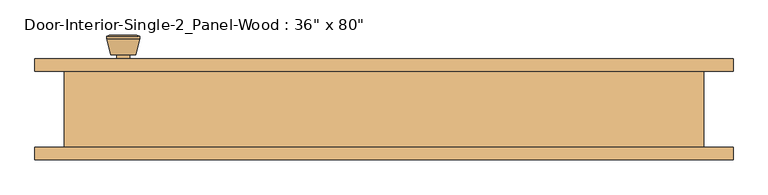
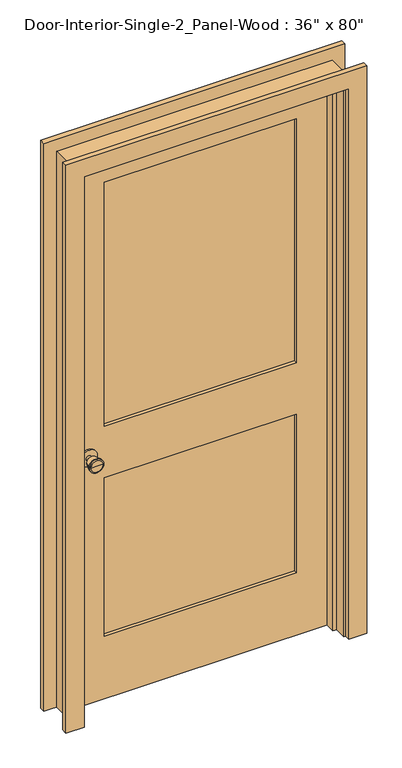
"""IFC4 building model written with IfcOpenShell, lengths in millimetres: door geometry."""

from ifc_helpers import new_model, si_unit, point, frame, frame_2d, origin, place, context, project, spatial, polyline, circle_curve, trimmed, segment, composite_curve, outline, extrude, faceted_brep, source, transform, mapped, element, save
from ifc_brep_helpers import plane_surface, cylinder_surface, revolved_surface, advanced_brep


def door_29124af5(model_context):
    return source(origin(), model_context, "Body", "SolidModel", [
        advanced_brep(
        [(-393.7, 13.05, 914.4), (-383.7, 13.05, 914.4), (-403.7, 13.05, 914.4), (-373.2241324, -35.95, 914.4), (-393.7, -35.95, 914.4), (-414.1758676, -35.95, 914.4), (-368.7, -34.1221319, 914.4), (-418.7, -34.1221319, 914.4), (-368.7, -30.6584537, 914.4), (-418.7, -30.6584537, 914.4), (-375.063764, -5.95, 914.4), (-412.336236, -5.95, 914.4), (-383.7, -5.95, 914.4), (-403.7, -5.95, 914.4)],
        [
            (0, 1),
            (1, 2, circle_curve(frame((-393.7, 13.05, 914.4), z_axis=(0.0, 1.0, 0.0), x_axis=(-1.0, 0.0, 0.0)), 10.0)),
            (2, 0),
            (2, 1, circle_curve(frame((-393.7, 13.05, 914.4), z_axis=(0.0, 1.0, 0.0), x_axis=(-1.0, 0.0, 0.0)), 10.0)),
            (3, 4),
            (4, 5),
            (5, 3, circle_curve(frame((-393.7, -35.95, 914.4), z_axis=(0.0, -1.0, 0.0), x_axis=(-1.0, 0.0, 0.0)), 20.4758676)),
            (3, 5, circle_curve(frame((-393.7, -35.95, 914.4), z_axis=(0.0, -1.0, 0.0), x_axis=(-1.0, 0.0, 0.0)), 20.4758676)),
            (6, 3),
            (5, 7),
            (7, 6, circle_curve(frame((-393.7, -34.1221319, 914.4), z_axis=(0.0, -1.0, 0.0), x_axis=(-1.0, 0.0, 0.0)), 25.0)),
            (6, 7, circle_curve(frame((-393.7, -34.1221319, 914.4), z_axis=(0.0, -1.0, 0.0), x_axis=(-1.0, 0.0, 0.0)), 25.0)),
            (8, 6),
            (7, 9),
            (9, 8, circle_curve(frame((-393.7, -30.6584537, 914.4), z_axis=(0.0, -1.0, 0.0), x_axis=(-1.0, 0.0, 0.0)), 25.0)),
            (8, 9, circle_curve(frame((-393.7, -30.6584537, 914.4), z_axis=(0.0, -1.0, 0.0), x_axis=(-1.0, 0.0, 0.0)), 25.0)),
            (10, 8),
            (9, 11),
            (11, 10, circle_curve(frame((-393.7, -5.95, 914.4), z_axis=(0.0, -1.0, 0.0), x_axis=(-1.0, 0.0, 0.0)), 18.636236)),
            (10, 11, circle_curve(frame((-393.7, -5.95, 914.4), z_axis=(0.0, -1.0, 0.0), x_axis=(-1.0, 0.0, 0.0)), 18.636236)),
            (12, 10),
            (11, 13),
            (13, 12, circle_curve(frame((-393.7, -5.95, 914.4), z_axis=(0.0, -1.0, 0.0), x_axis=(-1.0, 0.0, 0.0)), 10.0)),
            (12, 13, circle_curve(frame((-393.7, -5.95, 914.4), z_axis=(0.0, -1.0, 0.0), x_axis=(-1.0, 0.0, 0.0)), 10.0)),
            (1, 12),
            (13, 2),
        ],
        [
            plane_surface(frame((-393.7, 13.05, 914.4), z_axis=(0.0, 1.0, 0.0), x_axis=(-1.0, 0.0, 0.0))),
            plane_surface(frame((-393.7, -35.95, 914.4), z_axis=(0.0, -1.0, 0.0), x_axis=(-1.0, 0.0, 0.0))),
            revolved_surface(polyline([(-414.1758676, -35.95, 914.4), (-418.7, -34.1221319, 914.4)]), (-393.7, 13.05, 914.4), (0.0, 1.0, 0.0)),
            cylinder_surface(frame((-393.7, 13.05, 914.4), z_axis=(0.0, 1.0, 0.0), x_axis=(-1.0, 0.0, 0.0)), 25.0),
            revolved_surface(polyline([(-418.7, -30.6584537, 914.4), (-412.336236, -5.95, 914.4)]), (-393.7, 13.05, 914.4), (0.0, 1.0, 0.0)),
            plane_surface(frame((-393.7, -5.95, 914.4), z_axis=(0.0, 1.0, 0.0), x_axis=(-1.0, 0.0, 0.0))),
            cylinder_surface(frame((-393.7, 13.05, 914.4), z_axis=(0.0, 1.0, 0.0), x_axis=(-1.0, 0.0, 0.0)), 10.0),
        ],
        [
            (0, [[1, 2, 3]]),
            (0, [[-3, 4, -1]]),
            (1, [[5, 6, 7]]),
            (1, [[-6, -5, 8]]),
            (2, [[9, -7, 10, 11]]),
            (2, [[-10, -8, -9, 12]]),
            (3, [[13, -11, 14, 15]]),
            (3, [[-14, -12, -13, 16]]),
            (4, [[17, -15, 18, 19]]),
            (4, [[-18, -16, -17, 20]]),
            (5, [[21, -19, 22, 23]]),
            (5, [[-22, -20, -21, 24]]),
            (6, [[25, -23, 26, -2]]),
            (6, [[-26, -24, -25, -4]]),
        ],
    ),
        extrude(outline(composite_curve([segment(trimmed(circle_curve(frame_2d((914.4, -393.7)), 30.0), [point((914.4, -423.7))], [point((914.4, -363.7))], False, "CARTESIAN"), True, "CONTINUOUS"), segment(trimmed(circle_curve(frame_2d((914.4, -393.7)), 30.0), [point((914.4, -363.7))], [point((914.4, -423.7))], False, "CARTESIAN"), True, "CONTINUOUS")], self_intersect=False)), frame((0.0, 13.05, 0.0), z_axis=(0.0, 1.0, 0.0), x_axis=(0.0, 0.0, 1.0)), (0.0, 0.0, 1.0), 6.0),
        advanced_brep(
        [(-393.7, 59.975, 914.4), (-403.7, 59.975, 914.4), (-383.7, 59.975, 914.4), (-373.2241324, 108.975, 914.4), (-414.1758676, 108.975, 914.4), (-393.7, 108.975, 914.4), (-368.7, 107.1471319, 914.4), (-418.7, 107.1471319, 914.4), (-368.7, 103.6834537, 914.4), (-418.7, 103.6834537, 914.4), (-375.063764, 78.975, 914.4), (-412.336236, 78.975, 914.4), (-383.7, 78.975, 914.4), (-403.7, 78.975, 914.4)],
        [
            (0, 1),
            (1, 2, circle_curve(frame((-393.7, 59.975, 914.4), z_axis=(0.0, -1.0, 0.0), x_axis=(-1.0, 0.0, 0.0)), 10.0)),
            (2, 0),
            (2, 1, circle_curve(frame((-393.7, 59.975, 914.4), z_axis=(0.0, -1.0, 0.0), x_axis=(-1.0, 0.0, 0.0)), 10.0)),
            (3, 4, circle_curve(frame((-393.7, 108.975, 914.4), z_axis=(0.0, 1.0, 0.0), x_axis=(-1.0, 0.0, 0.0)), 20.4758676)),
            (4, 5),
            (5, 3),
            (4, 3, circle_curve(frame((-393.7, 108.975, 914.4), z_axis=(0.0, 1.0, 0.0), x_axis=(-1.0, 0.0, 0.0)), 20.4758676)),
            (6, 7, circle_curve(frame((-393.7, 107.1471319, 914.4), z_axis=(0.0, 1.0, 0.0), x_axis=(-1.0, 0.0, 0.0)), 25.0)),
            (7, 4),
            (3, 6),
            (7, 6, circle_curve(frame((-393.7, 107.1471319, 914.4), z_axis=(0.0, 1.0, 0.0), x_axis=(-1.0, 0.0, 0.0)), 25.0)),
            (8, 9, circle_curve(frame((-393.7, 103.6834537, 914.4), z_axis=(0.0, 1.0, 0.0), x_axis=(-1.0, 0.0, 0.0)), 25.0)),
            (9, 7),
            (6, 8),
            (9, 8, circle_curve(frame((-393.7, 103.6834537, 914.4), z_axis=(0.0, 1.0, 0.0), x_axis=(-1.0, 0.0, 0.0)), 25.0)),
            (10, 11, circle_curve(frame((-393.7, 78.975, 914.4), z_axis=(0.0, 1.0, 0.0), x_axis=(-1.0, 0.0, 0.0)), 18.636236)),
            (11, 9),
            (8, 10),
            (11, 10, circle_curve(frame((-393.7, 78.975, 914.4), z_axis=(0.0, 1.0, 0.0), x_axis=(-1.0, 0.0, 0.0)), 18.636236)),
            (12, 13, circle_curve(frame((-393.7, 78.975, 914.4), z_axis=(0.0, 1.0, 0.0), x_axis=(-1.0, 0.0, 0.0)), 10.0)),
            (13, 11),
            (10, 12),
            (13, 12, circle_curve(frame((-393.7, 78.975, 914.4), z_axis=(0.0, 1.0, 0.0), x_axis=(-1.0, 0.0, 0.0)), 10.0)),
            (1, 13),
            (12, 2),
        ],
        [
            plane_surface(frame((-393.7, 59.975, 914.4), z_axis=(0.0, -1.0, 0.0), x_axis=(-1.0, 0.0, 0.0))),
            plane_surface(frame((-393.7, 108.975, 914.4), z_axis=(0.0, 1.0, 0.0), x_axis=(-1.0, 0.0, 0.0))),
            revolved_surface(polyline([(-414.1758676, 108.975, 914.4), (-418.7, 107.1471319, 914.4)]), (-393.7, 59.975, 914.4), (0.0, -1.0, 0.0)),
            cylinder_surface(frame((-393.7, 59.975, 914.4), z_axis=(0.0, -1.0, 0.0), x_axis=(-1.0, 0.0, 0.0)), 25.0),
            revolved_surface(polyline([(-418.7, 103.6834537, 914.4), (-412.336236, 78.975, 914.4)]), (-393.7, 59.975, 914.4), (0.0, -1.0, 0.0)),
            plane_surface(frame((-393.7, 78.975, 914.4), z_axis=(0.0, -1.0, 0.0), x_axis=(-1.0, 0.0, 0.0))),
            cylinder_surface(frame((-393.7, 59.975, 914.4), z_axis=(0.0, -1.0, 0.0), x_axis=(-1.0, 0.0, 0.0)), 10.0),
        ],
        [
            (0, [[1, 2, 3]]),
            (0, [[-3, 4, -1]]),
            (1, [[5, 6, 7]]),
            (1, [[8, -7, -6]]),
            (2, [[9, 10, -5, 11]]),
            (2, [[12, -11, -8, -10]]),
            (3, [[13, 14, -9, 15]]),
            (3, [[16, -15, -12, -14]]),
            (4, [[17, 18, -13, 19]]),
            (4, [[20, -19, -16, -18]]),
            (5, [[21, 22, -17, 23]]),
            (5, [[24, -23, -20, -22]]),
            (6, [[-2, 25, -21, 26]]),
            (6, [[-4, -26, -24, -25]]),
        ],
    ),
        extrude(outline(composite_curve([segment(trimmed(circle_curve(frame_2d((914.4, -393.7)), 30.0), [point((914.4, -423.7))], [point((914.4, -363.7))], False, "CARTESIAN"), True, "CONTINUOUS"), segment(trimmed(circle_curve(frame_2d((914.4, -393.7)), 30.0), [point((914.4, -363.7))], [point((914.4, -423.7))], False, "CARTESIAN"), True, "CONTINUOUS")], self_intersect=False)), frame((0.0, 53.975, 0.0), z_axis=(0.0, 1.0, 0.0), x_axis=(0.0, 0.0, 1.0)), (0.0, 0.0, 1.0), 6.0),
        faceted_brep([(482.6, 53.975, 0.0), (482.6, -60.325, 0.0), (457.2, -60.325, 0.0), (457.2, -15.875, 0.0), (444.5, -15.875, 0.0), (444.5, 19.05, 0.0), (457.2, 19.05, 0.0), (457.2, 53.975, 0.0), (482.6, 53.975, 2057.4), (482.6, -60.325, 2057.4), (-482.6, -60.325, 2057.4), (-482.6, -60.325, 0.0), (-457.2, -60.325, 0.0), (-457.2, -60.325, 2032.0), (457.2, -60.325, 2032.0), (457.2, -15.875, 2032.0), (-457.2, -15.875, 2032.0), (-457.2, -15.875, 0.0), (-444.5, -15.875, 0.0), (-444.5, -15.875, 2019.3), (444.5, -15.875, 2019.3), (444.5, 19.05, 2019.3), (-444.5, 19.05, 2019.3), (-444.5, 19.05, 0.0), (-457.2, 19.05, 0.0), (-457.2, 19.05, 2032.0), (457.2, 19.05, 2032.0), (457.2, 53.975, 2032.0), (-457.2, 53.975, 2032.0), (-457.2, 53.975, 0.0), (-482.6, 53.975, 0.0), (-482.6, 53.975, 2057.4)], [[[0, 1, 2, 3, 4, 5, 6, 7]], [[1, 0, 8, 9]], [[2, 1, 9, 10, 11, 12, 13, 14]], [[3, 2, 14, 15]], [[4, 3, 15, 16, 17, 18, 19, 20]], [[5, 4, 20, 21]], [[6, 5, 21, 22, 23, 24, 25, 26]], [[7, 6, 26, 27]], [[0, 7, 27, 28, 29, 30, 31, 8]], [[9, 8, 31, 10]], [[15, 14, 13, 16]], [[21, 20, 19, 22]], [[27, 26, 25, 28]], [[30, 29, 24, 23, 18, 17, 12, 11]], [[10, 31, 30, 11]], [[16, 13, 12, 17]], [[22, 19, 18, 23]], [[28, 25, 24, 29]]]),
        extrude(outline(polyline([(2032.0, -457.2), (0.0, -457.2), (0.0, 457.2), (2032.0, 457.2), (2032.0, -457.2)]), holes=[polyline([(1912.9375, -336.55), (1912.9375, 336.55), (1009.65, 336.55), (1009.65, -336.55), (1912.9375, -336.55)]), polyline([(819.15, -336.55), (819.15, 336.55), (231.775, 336.55), (231.775, -336.55), (819.15, -336.55)])]), frame((0.0, 19.05, 0.0), z_axis=(0.0, 1.0, 0.0), x_axis=(0.0, 0.0, 1.0)), (0.0, 0.0, 1.0), 34.925),
        extrude(outline(polyline([(336.55, 30.6916667), (-336.55, 30.6916667), (-336.55, 42.3333333), (336.55, 42.3333333), (336.55, 30.6916667)])), frame((0.0, 0.0, 1009.65), z_axis=(0.0, 0.0, 1.0), x_axis=(1.0, 0.0, 0.0)), (0.0, 0.0, 1.0), 903.2875),
        extrude(outline(polyline([(336.55, 30.6916667), (-336.55, 30.6916667), (-336.55, 42.3333333), (336.55, 42.3333333), (336.55, 30.6916667)])), frame((0.0, 0.0, 231.775), z_axis=(0.0, 0.0, 1.0), x_axis=(1.0, 0.0, 0.0)), (0.0, 0.0, 1.0), 587.375),
        extrude(outline(polyline([(0.0, 463.55), (0.0, 527.05), (2101.85, 527.05), (2101.85, -527.05), (0.0, -527.05), (0.0, -463.55), (2038.35, -463.55), (2038.35, 463.55), (0.0, 463.55)])), frame((0.0, 53.975, 0.0), z_axis=(0.0, 1.0, 0.0), x_axis=(0.0, 0.0, 1.0)), (0.0, 0.0, 1.0), 19.05),
        extrude(outline(polyline([(0.0, 463.55), (0.0, 527.05), (2101.85, 527.05), (2101.85, -527.05), (0.0, -527.05), (0.0, -463.55), (2038.35, -463.55), (2038.35, 463.55), (0.0, 463.55)])), frame((0.0, -79.375, 0.0), z_axis=(0.0, 1.0, 0.0), x_axis=(0.0, 0.0, 1.0)), (0.0, 0.0, 1.0), 19.05),
    ])


if __name__ == "__main__":
    model = new_model("IFC4")
    model_context = context("Model", 3, world=origin())
    ifc_project = project(units=[si_unit("LENGTHUNIT", "METRE", prefix="MILLI")], contexts=[model_context])
    site = spatial("IfcSite", under=ifc_project)
    building = spatial("IfcBuilding", under=site)
    placement = place(None, origin())
    door_shape = door_29124af5(model_context)
    element("IfcDoor", 1, ObjectType="Door-Interior-Single-2_Panel-Wood : 36\" x 80\"", at=placement, inside=building, context=model_context, shape_type="MappedRepresentation", body=[
        mapped(door_shape, transform((0.0, 0.0, 0.0), x_axis=(1.0, 0.0, 0.0), y_axis=(0.0, 1.0, 0.0), z_axis=(0.0, 0.0, 1.0))),
    ])
    save(model, "model.ifc")

# Revit data of these elements
# Type "Door-Interior-Single-2_Panel-Wood : 36\" x 80\""
#   Type Mark = "9"
#   Assembly Code = "C1020300"
#   Analytic Construction = "Wooden"
#   Top Rail = 0' - 4 11/16"
#   Thickness = 0' - 1 3/8"
#   Thermal Resistance (R) = 2.5876 (h·ft²·°F)/BTU
#   Swing Angle [instance default] = 90.00°
#   Stiles = 0' - 4 3/4"
#   Rough Width = 3' - 2"
#   Rough Height = 6' - 9"
#   Lock Rail = 0' - 7 1/2"
#   Height = 6' - 8"
#   Width = 3' - 0"
#   Heat Transfer Coefficient (U) = 0.3865 BTU/(h·ft²·°F)
#   Bottom Rail = 0' - 9 1/8"
#   Trim Material = Cherry
#   Panel Material = Cherry
#   Frame Material = Cherry
#   Door Handle Material = Aluminum
#   Visual Light Transmittance = 0
#   Solar Heat Gain Coefficient = 0
#   Wall Closure = (empty or 0)
#   Function = (empty or 0)
# Element 1 (IfcDoor, "Door-Interior-Single-2_Panel-Wood : 36\" x 80\"")
#   Materials on its faces: "Cherry", "Aluminum"
# Materials
#   "Cherry": class "Wood", colour RGB 226 177 128, transparency 0, Description = "Prunus Serotina", Cost = 0
#   "Aluminum": class "Metal", colour RGB 247 247 247, transparency 0, Description = "Aluminum 6061", Cost = 0
